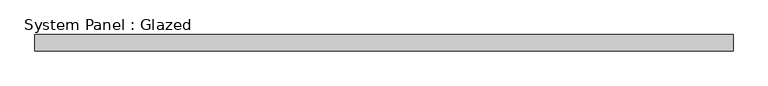
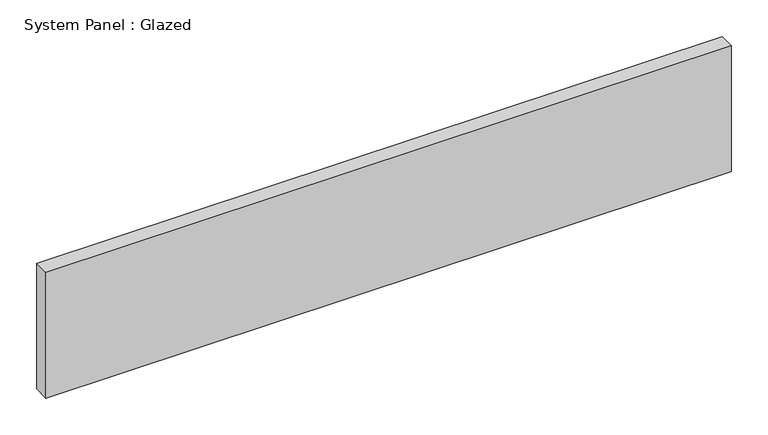
"""IFC4 building model written with IfcOpenShell, lengths in millimetres: plate geometry, System Panel : Glazed."""

from ifc_helpers import new_model, si_unit, origin, origin_with_axes, place, context, project, spatial, polyline, outline, extrude, source, transform, mapped, element, save


def system_panel_glazed_1d13bf28(model_context):
    return source(origin(), model_context, "Body", "SweptSolid", [
        extrude(outline(polyline([(539.75, 19.05), (-539.75, 19.05), (-539.75, 44.45), (539.75, 44.45), (539.75, 19.05)])), origin_with_axes(), (0.0, 0.0, 1.0), 209.55),
    ])


if __name__ == "__main__":
    model = new_model("IFC4")
    model_context = context("Model", 3, world=origin())
    ifc_project = project(units=[si_unit("LENGTHUNIT", "METRE", prefix="MILLI")], contexts=[model_context])
    site = spatial("IfcSite", under=ifc_project)
    building = spatial("IfcBuilding", under=site)
    placement = place(None, origin())
    system_panel_glazed_shape = system_panel_glazed_1d13bf28(model_context)
    element("IfcPlate", 1, ObjectType="System Panel : Glazed", at=placement, inside=building, context=model_context, shape_type="MappedRepresentation", body=[
        mapped(system_panel_glazed_shape, transform((0.0, 0.0, 0.0), x_axis=(1.0, 0.0, 0.0), y_axis=(0.0, 1.0, 0.0), z_axis=(0.0, 0.0, 1.0))),
    ])
    save(model, "model.ifc")

# Revit data of these elements
# Type "System Panel : Glazed"
#   Construction Type Id = "GSP4R"
#   Analytic Construction = "1/8 in Pilkington single glazing"
#   Visual Light Transmittance = 0.9
#   Solar Heat Gain Coefficient = 0.86
#   Heat Transfer Coefficient (U) = 1.18115 BTU/(h·ft²·°F)
#   Define Thermal Properties by = 1
# Element 1 (IfcPlate, "System Panel : Glazed")
#   Materials on its faces: "Glass"
# Materials
#   "Glass": class "Glass", colour RGB 0 128 192, transparency 0.75, Description = "Soda Lime Glass", Cost = 0
